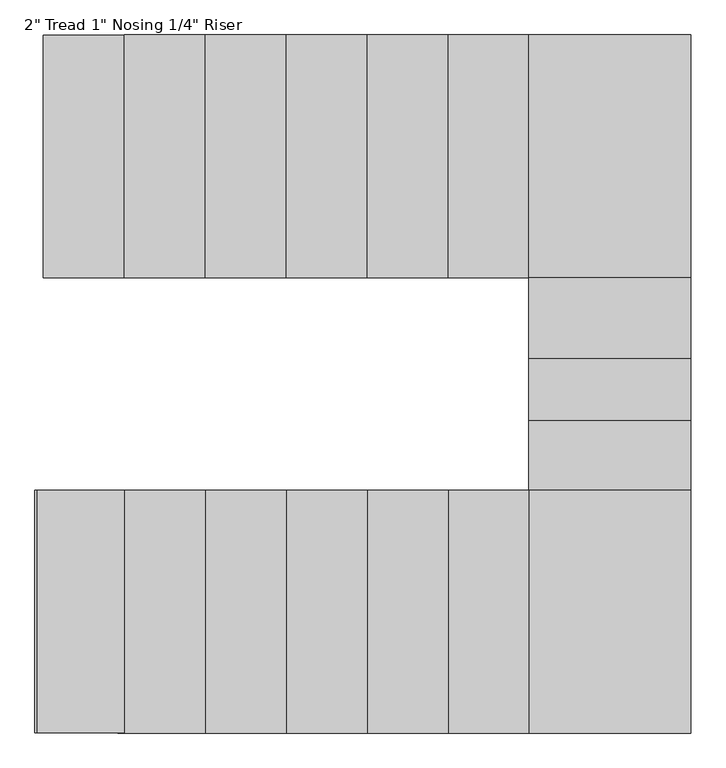
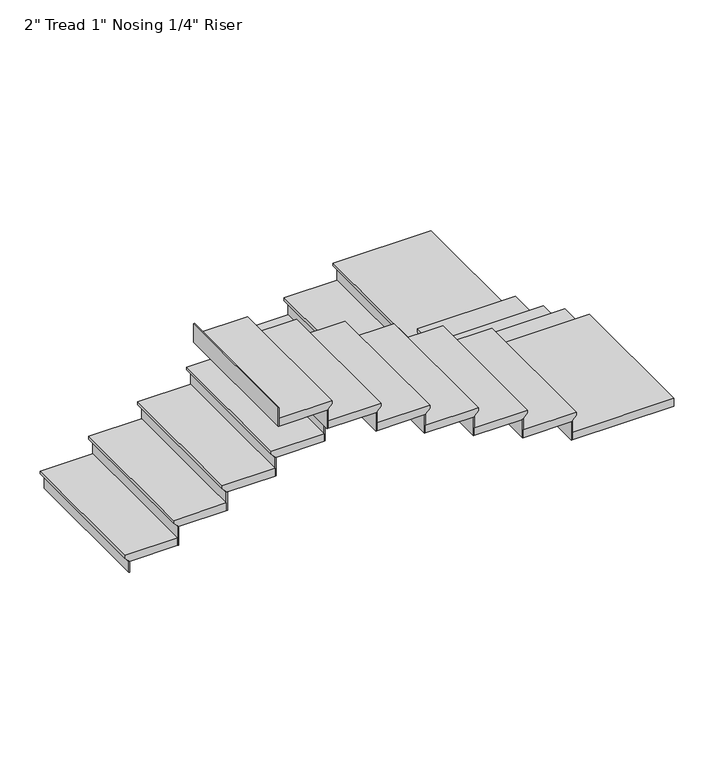
"""IFC4 building model written with IfcOpenShell, lengths in millimetres: stair flight geometry."""

from ifc_helpers import new_model, si_unit, origin, place, context, project, spatial, faceted_brep, source, transform, mapped, element, save


def stair_flight_8b794a03(model_context):
    return source(origin(), model_context, "Body", "Brep", [
        faceted_brep([(6477.0, 10054.8323212, 102.87), (6477.0, 10054.8323212, 121.92), (6477.0, 10969.2323212, 121.92), (6477.0, 10969.2323212, 102.87), (6502.4, 10054.8323212, 77.47), (6502.4, 10969.2323212, 77.47), (6807.2, 10054.8323212, 121.92), (6807.2, 10969.2323212, 121.92), (6502.4, 10969.2323212, 71.12), (6807.2, 10969.2323212, 71.12), (6807.2, 10054.8323212, 71.12), (6502.4, 10054.8323212, 71.12)], [[[0, 1, 2, 3]], [[4, 0, 3, 5]], [[2, 1, 6, 7]], [[8, 9, 10, 11]], [[2, 7, 9, 8, 5, 3]], [[8, 11, 4, 5]], [[6, 1, 0, 4, 11, 10]], [[7, 6, 10, 9]]]),
        faceted_brep([(6502.4, 10054.8323212, 71.12), (6502.4, 10054.8323212, 0.0), (6508.75, 10054.8323212, 0.0), (6508.75, 10054.8323212, 71.12), (6502.4, 10969.2323212, 71.12), (6508.75, 10969.2323212, 71.12), (6508.75, 10969.2323212, 0.0), (6502.4, 10969.2323212, 0.0)], [[[0, 1, 2, 3]], [[4, 5, 6, 7]], [[1, 0, 4, 7]], [[2, 1, 7, 6]], [[3, 2, 6, 5]], [[0, 3, 5, 4]]]),
        faceted_brep([(6807.2, 10054.8323212, 193.04), (6807.2, 10054.8323212, 71.12), (6813.55, 10054.8323212, 71.12), (6813.55, 10054.8323212, 193.04), (6807.2, 10969.2323212, 193.04), (6813.55, 10969.2323212, 193.04), (6813.55, 10969.2323212, 71.12), (6807.2, 10969.2323212, 71.12)], [[[0, 1, 2, 3]], [[4, 5, 6, 7]], [[1, 0, 4, 7]], [[2, 1, 7, 6]], [[3, 2, 6, 5]], [[0, 3, 5, 4]]]),
        faceted_brep([(6781.8, 10969.2323212, 243.84), (6781.8, 10054.8323212, 243.84), (7112.0, 10054.8323212, 243.84), (7112.0, 10969.2323212, 243.84), (6807.2, 10969.2323212, 193.04), (7112.0, 10969.2323212, 193.04), (7112.0, 10054.8323212, 193.04), (6807.2, 10054.8323212, 193.04), (6807.2, 10969.2323212, 199.39), (6781.8, 10969.2323212, 224.79), (6807.2, 10054.8323212, 199.39), (6781.8, 10054.8323212, 224.79)], [[[0, 1, 2, 3]], [[4, 5, 6, 7]], [[0, 3, 5, 4, 8, 9]], [[4, 7, 10, 8]], [[2, 1, 11, 10, 7, 6]], [[3, 2, 6, 5]], [[11, 1, 0, 9]], [[10, 11, 9, 8]]]),
        faceted_brep([(7112.0, 10054.8323212, 314.96), (7112.0, 10054.8323212, 193.04), (7118.35, 10054.8323212, 193.04), (7118.35, 10054.8323212, 314.96), (7112.0, 10969.2323212, 314.96), (7118.35, 10969.2323212, 314.96), (7118.35, 10969.2323212, 193.04), (7112.0, 10969.2323212, 193.04)], [[[0, 1, 2, 3]], [[4, 5, 6, 7]], [[1, 0, 4, 7]], [[2, 1, 7, 6]], [[3, 2, 6, 5]], [[0, 3, 5, 4]]]),
        faceted_brep([(7086.6, 10969.2323212, 365.76), (7086.6, 10054.8323212, 365.76), (7416.8, 10054.8323212, 365.76), (7416.8, 10969.2323212, 365.76), (7112.0, 10969.2323212, 314.96), (7416.8, 10969.2323212, 314.96), (7416.8, 10054.8323212, 314.96), (7112.0, 10054.8323212, 314.96), (7112.0, 10969.2323212, 321.31), (7086.6, 10969.2323212, 346.71), (7112.0, 10054.8323212, 321.31), (7086.6, 10054.8323212, 346.71)], [[[0, 1, 2, 3]], [[4, 5, 6, 7]], [[0, 3, 5, 4, 8, 9]], [[4, 7, 10, 8]], [[2, 1, 11, 10, 7, 6]], [[3, 2, 6, 5]], [[11, 1, 0, 9]], [[10, 11, 9, 8]]]),
        faceted_brep([(7416.8, 10054.8323212, 436.88), (7416.8, 10054.8323212, 314.96), (7423.15, 10054.8323212, 314.96), (7423.15, 10054.8323212, 436.88), (7416.8, 10969.2323212, 436.88), (7423.15, 10969.2323212, 436.88), (7423.15, 10969.2323212, 314.96), (7416.8, 10969.2323212, 314.96)], [[[0, 1, 2, 3]], [[4, 5, 6, 7]], [[1, 0, 4, 7]], [[2, 1, 7, 6]], [[3, 2, 6, 5]], [[0, 3, 5, 4]]]),
        faceted_brep([(7391.4, 10969.2323212, 487.68), (7391.4, 10054.8323212, 487.68), (7721.6, 10054.8323212, 487.68), (7721.6, 10969.2323212, 487.68), (7416.8, 10969.2323212, 436.88), (7721.6, 10969.2323212, 436.88), (7721.6, 10054.8323212, 436.88), (7416.8, 10054.8323212, 436.88), (7416.8, 10969.2323212, 443.23), (7391.4, 10969.2323212, 468.63), (7416.8, 10054.8323212, 443.23), (7391.4, 10054.8323212, 468.63)], [[[0, 1, 2, 3]], [[4, 5, 6, 7]], [[0, 3, 5, 4, 8, 9]], [[4, 7, 10, 8]], [[2, 1, 11, 10, 7, 6]], [[3, 2, 6, 5]], [[11, 1, 0, 9]], [[10, 11, 9, 8]]]),
        faceted_brep([(7721.6, 10054.8323212, 558.8), (7721.6, 10054.8323212, 436.88), (7727.95, 10054.8323212, 436.88), (7727.95, 10054.8323212, 558.8), (7721.6, 10969.2323212, 558.8), (7727.95, 10969.2323212, 558.8), (7727.95, 10969.2323212, 436.88), (7721.6, 10969.2323212, 436.88)], [[[0, 1, 2, 3]], [[4, 5, 6, 7]], [[1, 0, 4, 7]], [[2, 1, 7, 6]], [[3, 2, 6, 5]], [[0, 3, 5, 4]]]),
        faceted_brep([(7696.2, 10969.2323212, 609.6), (7696.2, 10054.8323212, 609.6), (8026.4, 10054.8323212, 609.6), (8026.4, 10969.2323212, 609.6), (7721.6, 10969.2323212, 558.8), (8026.4, 10969.2323212, 558.8), (8026.4, 10054.8323212, 558.8), (7721.6, 10054.8323212, 558.8), (7721.6, 10969.2323212, 565.15), (7696.2, 10969.2323212, 590.55), (7721.6, 10054.8323212, 565.15), (7696.2, 10054.8323212, 590.55)], [[[0, 1, 2, 3]], [[4, 5, 6, 7]], [[0, 3, 5, 4, 8, 9]], [[4, 7, 10, 8]], [[2, 1, 11, 10, 7, 6]], [[3, 2, 6, 5]], [[11, 1, 0, 9]], [[10, 11, 9, 8]]]),
        faceted_brep([(8026.4, 10054.8323212, 680.72), (8026.4, 10054.8323212, 558.8), (8032.75, 10054.8323212, 558.8), (8032.75, 10054.8323212, 680.72), (8026.4, 10969.2323212, 680.72), (8032.75, 10969.2323212, 680.72), (8032.75, 10969.2323212, 558.8), (8026.4, 10969.2323212, 558.8)], [[[0, 1, 2, 3]], [[4, 5, 6, 7]], [[1, 0, 4, 7]], [[2, 1, 7, 6]], [[3, 2, 6, 5]], [[0, 3, 5, 4]]]),
        faceted_brep([(8001.0, 10969.2323212, 731.52), (8001.0, 10054.8323212, 731.52), (8331.2, 10054.8323212, 731.52), (8331.2, 10969.2323212, 731.52), (8026.4, 10969.2323212, 680.72), (8331.2, 10969.2323212, 680.72), (8331.2, 10054.8323212, 680.72), (8026.4, 10054.8323212, 680.72), (8026.4, 10969.2323212, 687.07), (8001.0, 10969.2323212, 712.47), (8026.4, 10054.8323212, 687.07), (8001.0, 10054.8323212, 712.47)], [[[0, 1, 2, 3]], [[4, 5, 6, 7]], [[0, 3, 5, 4, 8, 9]], [[4, 7, 10, 8]], [[2, 1, 11, 10, 7, 6]], [[3, 2, 6, 5]], [[11, 1, 0, 9]], [[10, 11, 9, 8]]]),
        faceted_brep([(8331.2, 10054.8323212, 802.64), (8331.2, 10054.8323212, 680.72), (8337.55, 10054.8323212, 680.72), (8337.55, 10054.8323212, 802.64), (8331.2, 10969.2323212, 802.64), (8337.55, 10969.2323212, 802.64), (8337.55, 10969.2323212, 680.72), (8331.2, 10969.2323212, 680.72)], [[[0, 1, 2, 3]], [[4, 5, 6, 7]], [[1, 0, 4, 7]], [[2, 1, 7, 6]], [[3, 2, 6, 5]], [[0, 3, 5, 4]]]),
        faceted_brep([(8915.4, 10029.4323212, 853.44), (8915.4, 10969.2323212, 853.44), (8305.8, 10969.2323212, 853.44), (8305.8, 10029.4323212, 853.44), (8915.4, 10969.2323212, 802.64), (8915.4, 10029.4323212, 802.64), (8305.8, 10029.4323212, 802.64), (8305.8, 10054.8323212, 802.64), (8331.2, 10054.8323212, 802.64), (8331.2, 10969.2323212, 802.64), (8331.2, 10969.2323212, 808.99), (8305.8, 10969.2323212, 834.39), (8331.2, 10054.8323212, 808.99), (8305.8, 10054.8323212, 834.39)], [[[0, 1, 2, 3]], [[4, 5, 6, 7, 8, 9]], [[1, 0, 5, 4]], [[2, 1, 4, 9, 10, 11]], [[9, 8, 12, 10]], [[8, 7, 13, 12]], [[3, 2, 11, 13, 7, 6]], [[0, 3, 6, 5]], [[11, 10, 12, 13]]]),
        faceted_brep([(8305.8, 10029.4323212, 924.56), (8305.8, 10029.4323212, 802.64), (8305.8, 10023.0823212, 802.64), (8305.8, 10023.0823212, 924.56), (8915.4, 10029.4323212, 924.56), (8915.4, 10023.0823212, 924.56), (8915.4, 10023.0823212, 802.64), (8915.4, 10029.4323212, 802.64)], [[[0, 1, 2, 3]], [[4, 5, 6, 7]], [[1, 0, 4, 7]], [[2, 1, 7, 6]], [[3, 2, 6, 5]], [[0, 3, 5, 4]]]),
        faceted_brep([(8915.4, 10054.8323212, 975.36), (8305.8, 10054.8323212, 975.36), (8305.8, 9724.6323212, 975.36), (8915.4, 9724.6323212, 975.36), (8915.4, 10029.4323212, 924.56), (8915.4, 9724.6323212, 924.56), (8305.8, 9724.6323212, 924.56), (8305.8, 10029.4323212, 924.56), (8915.4, 10029.4323212, 930.91), (8915.4, 10054.8323212, 956.31), (8305.8, 10029.4323212, 930.91), (8305.8, 10054.8323212, 956.31)], [[[0, 1, 2, 3]], [[4, 5, 6, 7]], [[0, 3, 5, 4, 8, 9]], [[4, 7, 10, 8]], [[2, 1, 11, 10, 7, 6]], [[3, 2, 6, 5]], [[11, 1, 0, 9]], [[10, 11, 9, 8]]]),
        faceted_brep([(8305.8, 9724.6323212, 1046.48), (8305.8, 9724.6323212, 924.56), (8305.8, 9718.2823212, 924.56), (8305.8, 9718.2823212, 1046.48), (8915.4, 9724.6323212, 1046.48), (8915.4, 9718.2823212, 1046.48), (8915.4, 9718.2823212, 924.56), (8915.4, 9724.6323212, 924.56)], [[[0, 1, 2, 3]], [[4, 5, 6, 7]], [[1, 0, 4, 7]], [[2, 1, 7, 6]], [[3, 2, 6, 5]], [[0, 3, 5, 4]]]),
        faceted_brep([(8915.4, 9750.0323212, 1097.28), (8305.8, 9750.0323212, 1097.28), (8305.8, 9491.8832929, 1097.28), (8915.4, 9491.8832929, 1097.28), (8915.4, 9724.6323212, 1046.48), (8915.4, 9491.8832929, 1046.48), (8305.8, 9491.8832929, 1046.48), (8305.8, 9724.6323212, 1046.48), (8915.4, 9724.6323212, 1052.83), (8915.4, 9750.0323212, 1078.23), (8305.8, 9724.6323212, 1052.83), (8305.8, 9750.0323212, 1078.23)], [[[0, 1, 2, 3]], [[4, 5, 6, 7]], [[0, 3, 5, 4, 8, 9]], [[4, 7, 10, 8]], [[2, 1, 11, 10, 7, 6]], [[3, 2, 6, 5]], [[11, 1, 0, 9]], [[10, 11, 9, 8]]]),
        faceted_brep([(8305.8, 9491.8832929, 1168.4), (8305.8, 9491.8832929, 1046.48), (8305.8, 9485.5332929, 1046.48), (8305.8, 9485.5332929, 1168.4), (8915.4, 9491.8832929, 1168.4), (8915.4, 9485.5332929, 1168.4), (8915.4, 9485.5332929, 1046.48), (8915.4, 9491.8832929, 1046.48)], [[[0, 1, 2, 3]], [[4, 5, 6, 7]], [[1, 0, 4, 7]], [[2, 1, 7, 6]], [[3, 2, 6, 5]], [[0, 3, 5, 4]]]),
        faceted_brep([(8915.4, 9517.2832929, 1219.2), (8305.8, 9517.2832929, 1219.2), (8305.8, 9229.3323212, 1219.2), (8915.4, 9229.3323212, 1219.2), (8915.4, 9491.8832929, 1168.4), (8915.4, 9229.3323212, 1168.4), (8305.8, 9229.3323212, 1168.4), (8305.8, 9491.8832929, 1168.4), (8915.4, 9491.8832929, 1174.75), (8915.4, 9517.2832929, 1200.15), (8305.8, 9491.8832929, 1174.75), (8305.8, 9517.2832929, 1200.15)], [[[0, 1, 2, 3]], [[4, 5, 6, 7]], [[0, 3, 5, 4, 8, 9]], [[4, 7, 10, 8]], [[2, 1, 11, 10, 7, 6]], [[3, 2, 6, 5]], [[11, 1, 0, 9]], [[10, 11, 9, 8]]]),
        faceted_brep([(8305.8, 9229.3323212, 1290.32), (8305.8, 9229.3323212, 1168.4), (8305.8, 9222.9823212, 1168.4), (8305.8, 9222.9823212, 1290.32), (8915.4, 9229.3323212, 1290.32), (8915.4, 9222.9823212, 1290.32), (8915.4, 9222.9823212, 1168.4), (8915.4, 9229.3323212, 1168.4)], [[[0, 1, 2, 3]], [[4, 5, 6, 7]], [[1, 0, 4, 7]], [[2, 1, 7, 6]], [[3, 2, 6, 5]], [[0, 3, 5, 4]]]),
        faceted_brep([(8280.4, 8340.3323212, 1341.12), (8915.4, 8340.3323212, 1341.12), (8915.4, 9254.7323212, 1341.12), (8280.4, 9254.7323212, 1341.12), (8915.4, 8340.3323212, 1290.32), (8280.4, 8340.3323212, 1290.32), (8280.4, 9254.7323212, 1290.32), (8305.8, 9254.7323212, 1290.32), (8305.8, 9229.3323212, 1290.32), (8915.4, 9229.3323212, 1290.32), (8915.4, 9229.3323212, 1296.67), (8915.4, 9254.7323212, 1322.07), (8305.8, 9229.3323212, 1296.67), (8305.8, 9254.7323212, 1322.07)], [[[0, 1, 2, 3]], [[4, 5, 6, 7, 8, 9]], [[1, 0, 5, 4]], [[2, 1, 4, 9, 10, 11]], [[9, 8, 12, 10]], [[8, 7, 13, 12]], [[3, 2, 11, 13, 7, 6]], [[0, 3, 6, 5]], [[11, 10, 12, 13]]]),
        faceted_brep([(8280.4, 9254.7323212, 1412.24), (8280.4, 9254.7323212, 1290.32), (8274.05, 9254.7323212, 1290.32), (8274.05, 9254.7323212, 1412.24), (8280.4, 8340.3323212, 1412.24), (8274.05, 8340.3323212, 1412.24), (8274.05, 8340.3323212, 1290.32), (8280.4, 8340.3323212, 1290.32)], [[[0, 1, 2, 3]], [[4, 5, 6, 7]], [[1, 0, 4, 7]], [[2, 1, 7, 6]], [[3, 2, 6, 5]], [[0, 3, 5, 4]]]),
        faceted_brep([(8305.8, 8340.3323212, 1463.04), (8305.8, 9254.7323212, 1463.04), (7975.6, 9254.7323212, 1463.04), (7975.6, 8340.3323212, 1463.04), (8280.4, 8340.3323212, 1412.24), (7975.6, 8340.3323212, 1412.24), (7975.6, 9254.7323212, 1412.24), (8280.4, 9254.7323212, 1412.24), (8280.4, 8340.3323212, 1418.59), (8305.8, 8340.3323212, 1443.99), (8280.4, 9254.7323212, 1418.59), (8305.8, 9254.7323212, 1443.99)], [[[0, 1, 2, 3]], [[4, 5, 6, 7]], [[0, 3, 5, 4, 8, 9]], [[4, 7, 10, 8]], [[2, 1, 11, 10, 7, 6]], [[3, 2, 6, 5]], [[11, 1, 0, 9]], [[10, 11, 9, 8]]]),
        faceted_brep([(7975.6, 9254.7323212, 1534.16), (7975.6, 9254.7323212, 1412.24), (7969.25, 9254.7323212, 1412.24), (7969.25, 9254.7323212, 1534.16), (7975.6, 8340.3323212, 1534.16), (7969.25, 8340.3323212, 1534.16), (7969.25, 8340.3323212, 1412.24), (7975.6, 8340.3323212, 1412.24)], [[[0, 1, 2, 3]], [[4, 5, 6, 7]], [[1, 0, 4, 7]], [[2, 1, 7, 6]], [[3, 2, 6, 5]], [[0, 3, 5, 4]]]),
        faceted_brep([(8001.0, 8340.3323212, 1584.96), (8001.0, 9254.7323212, 1584.96), (7670.8, 9254.7323212, 1584.96), (7670.8, 8340.3323212, 1584.96), (7975.6, 8340.3323212, 1534.16), (7670.8, 8340.3323212, 1534.16), (7670.8, 9254.7323212, 1534.16), (7975.6, 9254.7323212, 1534.16), (7975.6, 8340.3323212, 1540.51), (8001.0, 8340.3323212, 1565.91), (7975.6, 9254.7323212, 1540.51), (8001.0, 9254.7323212, 1565.91)], [[[0, 1, 2, 3]], [[4, 5, 6, 7]], [[0, 3, 5, 4, 8, 9]], [[4, 7, 10, 8]], [[2, 1, 11, 10, 7, 6]], [[3, 2, 6, 5]], [[11, 1, 0, 9]], [[10, 11, 9, 8]]]),
        faceted_brep([(7670.8, 9254.7323212, 1656.08), (7670.8, 9254.7323212, 1534.16), (7664.45, 9254.7323212, 1534.16), (7664.45, 9254.7323212, 1656.08), (7670.8, 8340.3323212, 1656.08), (7664.45, 8340.3323212, 1656.08), (7664.45, 8340.3323212, 1534.16), (7670.8, 8340.3323212, 1534.16)], [[[0, 1, 2, 3]], [[4, 5, 6, 7]], [[1, 0, 4, 7]], [[2, 1, 7, 6]], [[3, 2, 6, 5]], [[0, 3, 5, 4]]]),
        faceted_brep([(7696.2, 8340.3323212, 1706.88), (7696.2, 9254.7323212, 1706.88), (7366.0, 9254.7323212, 1706.88), (7366.0, 8340.3323212, 1706.88), (7670.8, 8340.3323212, 1656.08), (7366.0, 8340.3323212, 1656.08), (7366.0, 9254.7323212, 1656.08), (7670.8, 9254.7323212, 1656.08), (7670.8, 8340.3323212, 1662.43), (7696.2, 8340.3323212, 1687.83), (7670.8, 9254.7323212, 1662.43), (7696.2, 9254.7323212, 1687.83)], [[[0, 1, 2, 3]], [[4, 5, 6, 7]], [[0, 3, 5, 4, 8, 9]], [[4, 7, 10, 8]], [[2, 1, 11, 10, 7, 6]], [[3, 2, 6, 5]], [[11, 1, 0, 9]], [[10, 11, 9, 8]]]),
        faceted_brep([(7366.0, 9254.7323212, 1778.0), (7366.0, 9254.7323212, 1656.08), (7359.65, 9254.7323212, 1656.08), (7359.65, 9254.7323212, 1778.0), (7366.0, 8340.3323212, 1778.0), (7359.65, 8340.3323212, 1778.0), (7359.65, 8340.3323212, 1656.08), (7366.0, 8340.3323212, 1656.08)], [[[0, 1, 2, 3]], [[4, 5, 6, 7]], [[1, 0, 4, 7]], [[2, 1, 7, 6]], [[3, 2, 6, 5]], [[0, 3, 5, 4]]]),
        faceted_brep([(7391.4, 8340.3323212, 1828.8), (7391.4, 9254.7323212, 1828.8), (7061.2, 9254.7323212, 1828.8), (7061.2, 8340.3323212, 1828.8), (7366.0, 8340.3323212, 1778.0), (7061.2, 8340.3323212, 1778.0), (7061.2, 9254.7323212, 1778.0), (7366.0, 9254.7323212, 1778.0), (7366.0, 8340.3323212, 1784.35), (7391.4, 8340.3323212, 1809.75), (7366.0, 9254.7323212, 1784.35), (7391.4, 9254.7323212, 1809.75)], [[[0, 1, 2, 3]], [[4, 5, 6, 7]], [[0, 3, 5, 4, 8, 9]], [[4, 7, 10, 8]], [[2, 1, 11, 10, 7, 6]], [[3, 2, 6, 5]], [[11, 1, 0, 9]], [[10, 11, 9, 8]]]),
        faceted_brep([(7061.2, 9254.7323212, 1899.92), (7061.2, 9254.7323212, 1778.0), (7054.85, 9254.7323212, 1778.0), (7054.85, 9254.7323212, 1899.92), (7061.2, 8340.3323212, 1899.92), (7054.85, 8340.3323212, 1899.92), (7054.85, 8340.3323212, 1778.0), (7061.2, 8340.3323212, 1778.0)], [[[0, 1, 2, 3]], [[4, 5, 6, 7]], [[1, 0, 4, 7]], [[2, 1, 7, 6]], [[3, 2, 6, 5]], [[0, 3, 5, 4]]]),
        faceted_brep([(7086.6, 8340.3323212, 1950.72), (7086.6, 9254.7323212, 1950.72), (6756.4, 9254.7323212, 1950.72), (6756.4, 8340.3323212, 1950.72), (7061.2, 8340.3323212, 1899.92), (6756.4, 8340.3323212, 1899.92), (6756.4, 9254.7323212, 1899.92), (7061.2, 9254.7323212, 1899.92), (7061.2, 8340.3323212, 1906.27), (7086.6, 8340.3323212, 1931.67), (7061.2, 9254.7323212, 1906.27), (7086.6, 9254.7323212, 1931.67)], [[[0, 1, 2, 3]], [[4, 5, 6, 7]], [[0, 3, 5, 4, 8, 9]], [[4, 7, 10, 8]], [[2, 1, 11, 10, 7, 6]], [[3, 2, 6, 5]], [[11, 1, 0, 9]], [[10, 11, 9, 8]]]),
        faceted_brep([(6756.4, 9254.7323212, 2021.84), (6756.4, 9254.7323212, 1899.92), (6750.05, 9254.7323212, 1899.92), (6750.05, 9254.7323212, 2021.84), (6756.4, 8340.3323212, 2021.84), (6750.05, 8340.3323212, 2021.84), (6750.05, 8340.3323212, 1899.92), (6756.4, 8340.3323212, 1899.92)], [[[0, 1, 2, 3]], [[4, 5, 6, 7]], [[1, 0, 4, 7]], [[2, 1, 7, 6]], [[3, 2, 6, 5]], [[0, 3, 5, 4]]]),
        faceted_brep([(6451.6, 9254.7323212, 2143.76), (6451.6, 9254.7323212, 2021.84), (6445.25, 9254.7323212, 2021.84), (6445.25, 9254.7323212, 2143.76), (6451.6, 8340.3323212, 2143.76), (6445.25, 8340.3323212, 2143.76), (6445.25, 8340.3323212, 2021.84), (6451.6, 8340.3323212, 2021.84)], [[[0, 1, 2, 3]], [[4, 5, 6, 7]], [[1, 0, 4, 7]], [[2, 1, 7, 6]], [[3, 2, 6, 5]], [[0, 3, 5, 4]]]),
        faceted_brep([(6781.8, 8340.3323212, 2072.64), (6781.8, 9254.7323212, 2072.64), (6451.6, 9254.7323212, 2072.64), (6451.6, 8340.3323212, 2072.64), (6756.4, 8340.3323212, 2021.84), (6451.6, 8340.3323212, 2021.84), (6451.6, 9254.7323212, 2021.84), (6756.4, 9254.7323212, 2021.84), (6756.4, 8340.3323212, 2028.19), (6781.8, 8340.3323212, 2053.59), (6756.4, 9254.7323212, 2028.19), (6781.8, 9254.7323212, 2053.59)], [[[0, 1, 2, 3]], [[4, 5, 6, 7]], [[0, 3, 5, 4, 8, 9]], [[4, 7, 10, 8]], [[2, 1, 11, 10, 7, 6]], [[3, 2, 6, 5]], [[11, 1, 0, 9]], [[10, 11, 9, 8]]]),
    ])


if __name__ == "__main__":
    model = new_model("IFC4")
    model_context = context("Model", 3, world=origin())
    ifc_project = project(units=[si_unit("LENGTHUNIT", "METRE", prefix="MILLI")], contexts=[model_context])
    site = spatial("IfcSite", under=ifc_project)
    building = spatial("IfcBuilding", under=site)
    placement = place(None, origin())
    stair_flight_shape = stair_flight_8b794a03(model_context)
    element("IfcStairFlight", 1, ObjectType="2\" Tread 1\" Nosing 1/4\" Riser", at=placement, inside=building, context=model_context, shape_type="MappedRepresentation", body=[
        mapped(stair_flight_shape, transform((0.0, 0.0, 0.0), x_axis=(1.0, 0.0, 0.0), y_axis=(0.0, 1.0, 0.0), z_axis=(0.0, 0.0, 1.0))),
    ])
    save(model, "model.ifc")
